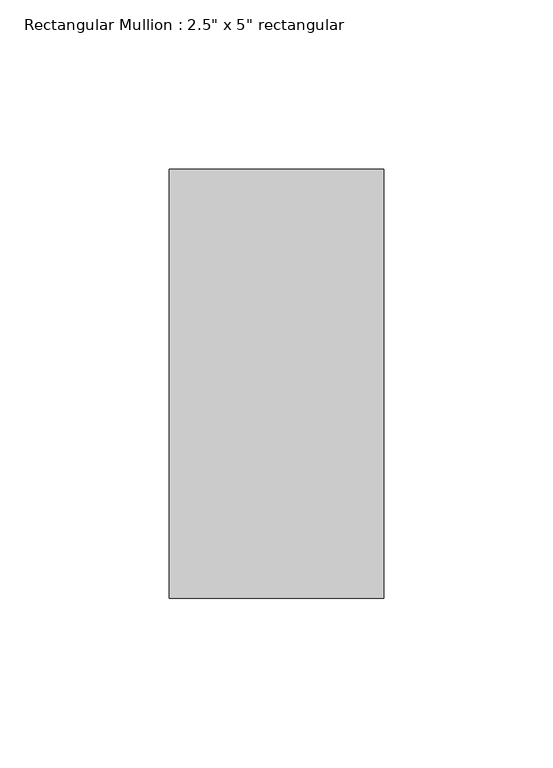
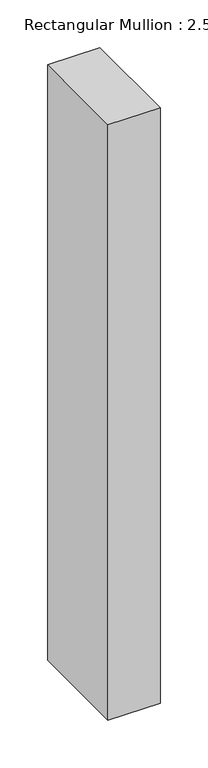
"""IFC4 building model written with IfcOpenShell, lengths in millimetres: member geometry."""

from ifc_helpers import new_model, si_unit, frame, origin, place, context, project, spatial, polyline, outline, extrude, source, transform, mapped, element, save


def member_a05a67d1(model_context):
    return source(origin(), model_context, "Body", "SweptSolid", [
        extrude(outline(polyline([(0.0, 63.5), (0.0, -63.5), (-63.5, -63.5), (-63.5, 63.5), (0.0, 63.5)])), frame((0.0, 0.0, -764.1166667), z_axis=(0.0, 0.0, 1.0), x_axis=(1.0, 0.0, 0.0)), (0.0, 0.0, 1.0), 764.1166667),
    ])


if __name__ == "__main__":
    model = new_model("IFC4")
    model_context = context("Model", 3, world=origin())
    ifc_project = project(units=[si_unit("LENGTHUNIT", "METRE", prefix="MILLI")], contexts=[model_context])
    site = spatial("IfcSite", under=ifc_project)
    building = spatial("IfcBuilding", under=site)
    placement = place(None, origin())
    member_shape = member_a05a67d1(model_context)
    element("IfcMember", 1, ObjectType="Rectangular Mullion : 2.5\" x 5\" rectangular", at=placement, inside=building, context=model_context, shape_type="MappedRepresentation", body=[
        mapped(member_shape, transform((0.0, 0.0, 0.0), x_axis=(1.0, 0.0, 0.0), y_axis=(0.0, 1.0, 0.0), z_axis=(0.0, 0.0, 1.0))),
    ])
    save(model, "model.ifc")

# Revit data of these elements
# Type "Rectangular Mullion : 2.5\" x 5\" rectangular"
#   built-in parameter 1007304 = 0.416667 (stored number, unit not read)
#   built-in parameter 1007301 = 0.104167 (stored number, unit not read)
#   built-in parameter 1007300 = 0.104167 (stored number, unit not read)
# Element 1 (IfcMember, "Rectangular Mullion : 2.5\" x 5\" rectangular")
#   Materials on its faces: "Aluminum"
# Materials
#   "Aluminum": class "Metal", colour RGB 247 247 247, transparency 0, Description = "Aluminum 6061", Cost = 0
